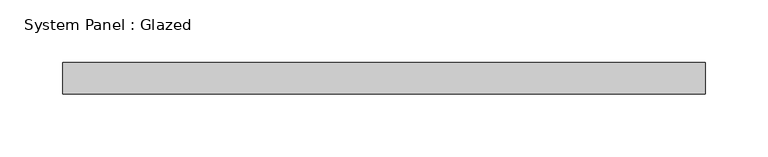
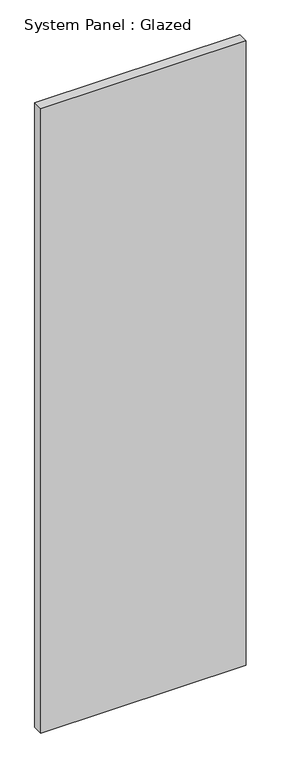
"""IFC4 building model written with IfcOpenShell, lengths in millimetres: plate geometry, System Panel : Glazed."""

from ifc_helpers import new_model, si_unit, origin, origin_with_axes, place, context, project, spatial, polyline, outline, extrude, source, transform, mapped, element, save


def system_panel_glazed_0947b60d(model_context):
    return source(origin(), model_context, "Body", "SweptSolid", [
        extrude(outline(polyline([(257.175, 19.05), (-257.175, 19.05), (-257.175, 44.45), (257.175, 44.45), (257.175, 19.05)])), origin_with_axes(), (0.0, 0.0, 1.0), 1652.2221241),
    ])


if __name__ == "__main__":
    model = new_model("IFC4")
    model_context = context("Model", 3, world=origin())
    ifc_project = project(units=[si_unit("LENGTHUNIT", "METRE", prefix="MILLI")], contexts=[model_context])
    site = spatial("IfcSite", under=ifc_project)
    building = spatial("IfcBuilding", under=site)
    placement = place(None, origin())
    system_panel_glazed_shape = system_panel_glazed_0947b60d(model_context)
    element("IfcPlate", 1, ObjectType="System Panel : Glazed", at=placement, inside=building, context=model_context, shape_type="MappedRepresentation", body=[
        mapped(system_panel_glazed_shape, transform((0.0, 0.0, 0.0), x_axis=(1.0, 0.0, 0.0), y_axis=(0.0, 1.0, 0.0), z_axis=(0.0, 0.0, 1.0))),
    ])
    save(model, "model.ifc")

# Revit data of these elements
# Type "System Panel : Glazed"
#   Construction Type Id = "GSP4R"
#   Analytic Construction = "1/8 in Pilkington single glazing"
#   Visual Light Transmittance = 0.9
#   Solar Heat Gain Coefficient = 0.86
#   Heat Transfer Coefficient (U) = 1.18115 BTU/(h·ft²·°F)
#   Define Thermal Properties by = 1
# Element 1 (IfcPlate, "System Panel : Glazed")
#   Materials on its faces: "Glass"
# Materials
#   "Glass": class "Glass", colour RGB 0 128 192, transparency 0.75, Description = "Soda Lime Glass", Cost = 0
